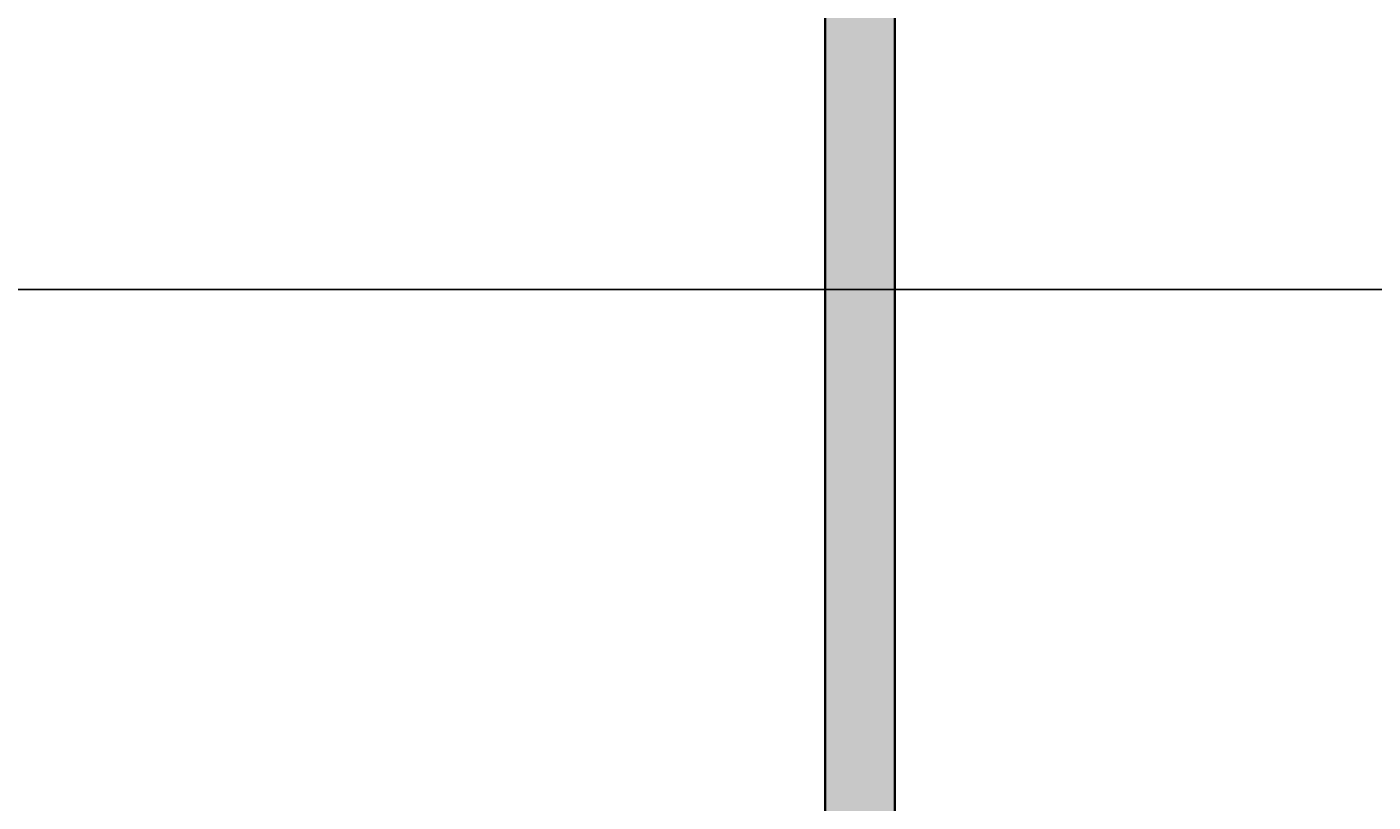
# Model space of a CAD drawing. Units: inches. Extents: x 1998 to 2588, y 1139 to 1977.
# Tile 5 of 134: x 2036 to 2075, y 1598 to 1620. Entities that reach past the tile are written whole.
import ezdxf

# ---------------------------------------------------------------- set-up
doc = ezdxf.new("R2010")
doc.units = ezdxf.units.IN
for name, color, linetype, lineweight in [('A-ANNO-DIMS', 2, 'Continuous', 18), ('A-WALL-PATT', 252, 'Continuous', 13), ('WALL', 200, 'Continuous', 35)]:
    doc.layers.add(name, color=color, linetype=linetype, lineweight=lineweight)
doc.styles.get("Standard").update_dxf_attribs({"font": 'arial.ttf'})
doc.dimstyles.get("Standard").update_dxf_attribs({"dimtxt": 0.18, "dimasz": 0.18, "dimexe": 0.18, "dimexo": 0.0625, "dimgap": 0.09, "dimtad": 0, "dimtih": 1, "dimtoh": 1, "dimdec": 4, "dimzin": 0, "dimdsep": 46, "dimtxsty": 'Standard', "dimcen": 0.09, "dimadec": 0, "dimazin": 0, "dimtfac": 1, "dimtdec": 4, "dimtofl": 0, "dimtmove": 0, "dimatfit": 3, "dimfxl": 1, "dimtolj": 1, "dimtzin": 0, "dimarcsym": 0})

# ---------------------------------------------------------------- blocks, each defined once
blk = doc.blocks.new('*D30')
at = {"layer": 'A-ANNO-DIMS', "color": 0, "lineweight": -2, "transparency": 16777216}
for p, q in [((2407.91, 1636.732), (1997.843, 1636.732)), ((1998.023, 1636.552), (1998.023, 1615.913)), ((1998.023, 1594.912), (1998.023, 1615.552)), ((2407.91, 1594.732), (1997.843, 1594.732))]:
    blk.add_line(p, q, dxfattribs=at)
at = {"layer": 'A-ANNO-DIMS', "color": 0, "transparency": 16777216}
for points in [[(1997.993, 1636.552), (1998.053, 1636.552), (1998.023, 1636.732)], [(1997.993, 1594.912), (1998.053, 1594.912), (1998.023, 1594.732)]]:
    blk.add_solid(points, dxfattribs=at)
at = {"layer": 'Defpoints', "color": 0, "transparency": 16777216}
for p in [(1998.023, 1636.732), (2407.973, 1636.732), (2407.973, 1594.732)]:
    blk.add_point(p, dxfattribs=at)
at = {"layer": 'A-ANNO-DIMS', "color": 0, "transparency": 16777216, "insert": (1998.023, 1615.732), "char_height": 0.18, "attachment_point": 5}
blk.add_mtext('\\A1;42', dxfattribs=at)
blk = doc.blocks.new('*D35')
at = {"layer": 'A-ANNO-DIMS', "color": 0, "lineweight": -2, "transparency": 16777216}
for p, q in [((2148.392, 1612.732), (1997.843, 1612.732)), ((1998.023, 1612.552), (1998.023, 1600.913)), ((1998.023, 1588.912), (1998.023, 1600.552)), ((2148.392, 1588.732), (1997.843, 1588.732))]:
    blk.add_line(p, q, dxfattribs=at)
at = {"layer": 'A-ANNO-DIMS', "color": 0, "transparency": 16777216}
for points in [[(1997.993, 1612.552), (1998.053, 1612.552), (1998.023, 1612.732)], [(1997.993, 1588.912), (1998.053, 1588.912), (1998.023, 1588.732)]]:
    blk.add_solid(points, dxfattribs=at)
at = {"layer": 'Defpoints', "color": 0, "transparency": 16777216}
for p in [(1998.023, 1612.732), (2148.455, 1612.732), (2148.455, 1588.732)]:
    blk.add_point(p, dxfattribs=at)
at = {"layer": 'A-ANNO-DIMS', "color": 0, "transparency": 16777216, "insert": (1998.023, 1600.732), "char_height": 0.18, "attachment_point": 5}
blk.add_mtext('\\A1;24', dxfattribs=at)
blk = doc.blocks.new('*D38')
at = {"layer": 'A-ANNO-DIMS', "color": 0, "lineweight": -2, "transparency": 16777216}
for p, q in [((2197.387, 1663.247), (1997.843, 1663.247)), ((1998.023, 1663.067), (1998.023, 1638.171)), ((1998.023, 1612.912), (1998.023, 1637.808)), ((2197.387, 1612.732), (1997.843, 1612.732))]:
    blk.add_line(p, q, dxfattribs=at)
at = {"layer": 'A-ANNO-DIMS', "color": 0, "transparency": 16777216}
for points in [[(1997.993, 1663.067), (1998.053, 1663.067), (1998.023, 1663.247)], [(1997.993, 1612.912), (1998.053, 1612.912), (1998.023, 1612.732)]]:
    blk.add_solid(points, dxfattribs=at)
at = {"layer": 'Defpoints', "color": 0, "transparency": 16777216}
for p in [(1998.023, 1663.247), (2197.45, 1663.247), (2197.45, 1612.732)]:
    blk.add_point(p, dxfattribs=at)
at = {"layer": 'A-ANNO-DIMS', "color": 0, "transparency": 16777216, "insert": (1998.023, 1637.99), "char_height": 0.18, "attachment_point": 5}
blk.add_mtext('\\A1;50.51', dxfattribs=at)

msp = doc.modelspace()

# ---------------------------------------------------------------- hatches: boundary and pattern name
at = {"layer": 'A-WALL-PATT'}
h = msp.add_hatch(color=256, dxfattribs=at)
h.dxf.hatch_style = 1
h.paths.add_polyline_path([(2227.4729, 1911.2324), (2222.9729, 1911.2324), (2222.9729, 1888.7324), (2227.4729, 1888.7324)])
h.paths.add_polyline_path([(2236.4493, 1870.3636), (2236.4493, 1875.2324), (2234.4125, 1875.2324), (2234.4125, 1868.3278), (2227.4729, 1868.3278), (2227.4729, 1866.2324), (2236.4493, 1866.2324)])
h.paths.add_polyline_path([(2330.0332, 1875.2324), (2263.9907, 1875.2324), (2263.9907, 1866.2324), (2330.0332, 1866.2324)])
h.paths.add_polyline_path([(2345.9729, 1906.7324), (2393.9729, 1906.7324), (2393.9729, 1882.7324), (2345.9729, 1882.7324), (2345.9729, 1878.2324), (2393.9729, 1878.2324), (2398.4729, 1878.2324), (2398.4729, 1882.7324), (2398.4729, 1911.2324), (2345.9729, 1911.2324), (2341.4729, 1911.2324), (2341.4729, 1866.2324), (2341.4729, 1790.0412), (2345.9729, 1790.0412), (2345.9729, 1875.2324)])
h.paths.add_polyline_path([(2398.4729, 1878.2324), (2393.9729, 1878.2324), (2393.9729, 1798.2324), (2393.9729, 1793.7324), (2398.4729, 1793.7324)], flags=17)
h.paths.add_polyline_path([(2393.9729, 1798.2324), (2375.7311, 1798.2324, -0.005968), (2375.7384, 1797.6146), (2375.7384, 1793.7324), (2393.9729, 1793.7324)], flags=17)
h.paths.add_polyline_path([(2349.8569, 1797.6146), (2349.8569, 1798.2324), (2345.9729, 1798.2324), (2345.9729, 1793.7324), (2349.8569, 1793.7324)], flags=17)
h.paths.add_polyline_path([(2398.4729, 1793.7324), (2393.9729, 1793.7324), (2393.9729, 1790.0412), (2398.4729, 1790.0412)], flags=17)
h.paths.add_polyline_path([(2527.4729, 1882.7324), (2507.8006, 1882.7324), (2507.8006, 1878.2324), (2518.4729, 1878.2324), (2518.4729, 1759.7324), (2510.9729, 1759.7324), (2510.9729, 1755.2324), (2527.4729, 1755.2324)])
h.paths.add_polyline_path([(2487.396, 1882.7324), (2398.4729, 1882.7324), (2398.4729, 1878.2324), (2487.396, 1878.2324)])
h.paths.add_polyline_path([(2490.5682, 1759.7324), (2345.9729, 1759.7324), (2345.9729, 1755.2324), (2490.5682, 1755.2324)])
h.paths.add_polyline_path([(2398.4729, 1760.5844), (2398.3914, 1760.5844), (2393.9729, 1760.5844), (2393.9729, 1759.7324), (2398.4729, 1759.7324)])
h.paths.add_polyline_path([(2334.5332, 1759.7324), (2234.4125, 1759.7324), (2234.4125, 1755.2324), (2334.5332, 1755.2324)])
h.paths.add_polyline_path([(2345.9729, 1760.5844), (2341.5543, 1760.5844), (2341.4729, 1760.5844), (2341.4729, 1759.7324), (2345.9729, 1759.7324)])
h.paths.add_polyline_path([(2222.9729, 1759.7324), (2221.7204, 1759.7324), (2221.7204, 1755.2324), (2222.9729, 1755.2324)])
h.paths.add_polyline_path([(2061.4729, 1702.7324), (2059.4729, 1702.7324), (2059.4729, 1584.2324), (2061.4729, 1584.2324)])
h.paths.add_polyline_path([(2061.4729, 1584.2324), (2059.4729, 1584.2324), (2059.4729, 1470.2324), (2061.4729, 1470.2324)])
h.paths.add_polyline_path([(2510.9729, 1469.2927), (2501.9729, 1469.2927), (2501.9729, 1369.172), (2510.9729, 1369.172)])
h.paths.add_polyline_path([(2227.4729, 1369.7324), (2227.4729, 1417.7324), (2221.4126, 1417.7324), (2221.4126, 1413.2324), (2222.9729, 1413.2324), (2222.9729, 1293.2324), (2222.9729, 1285.137), (2227.4729, 1285.137)])

# ---------------------------------------------------------------- linework, layer by layer
at = {"layer": 'WALL'}
for p, q in [((2061.4729, 1473.2749), (2061.4729, 1705.7749)), ((2059.4729, 1470.2324), (2059.4729, 1702.7324))]:
    msp.add_line(p, q, dxfattribs=at)
msp.add_lwpolyline([(2059.4729, 1584.2324), (2061.4729, 1584.2324), (2061.4729, 1702.7324), (2059.4729, 1702.7324)], close=True, dxfattribs=at)

# ---------------------------------------------------------------- dimensions: what is measured, and where the dimension line sits
at = {"layer": 'A-ANNO-DIMS'}
for base, p1, p2, override, picture, middle in [((1998.0229, 1663.2466), (2197.4499, 1612.7324), (2197.4499, 1663.2466), {"dimdec": 2, "dimlfac": 1, "dimrnd": 0, "dimzin": 0, "dimdsep": 46, "dimlunit": 2}, '*D38', (1998.0229, 1637.9895)), ((1998.0229, 1636.7324), (2407.9729, 1594.7324), (2407.9729, 1636.7324), {"dimdec": 0, "dimlfac": 1, "dimrnd": 0, "dimzin": 0, "dimdsep": 46, "dimlunit": 2}, '*D30', (1998.0229, 1615.7324)), ((1998.0229, 1612.7324), (2148.4548, 1588.7324), (2148.4548, 1612.7324), {"dimdec": 0, "dimlfac": 1, "dimrnd": 0, "dimzin": 0, "dimdsep": 46, "dimlunit": 2}, '*D35', (1998.0229, 1600.7324))]:
    dim = msp.add_linear_dim(base=base, p1=p1, p2=p2, angle=90, dimstyle='Standard', override=override, dxfattribs=at)
    dim.commit()
    dim.dimension.update_dxf_attribs({"geometry": picture, "text_midpoint": middle})

doc.saveas('drawing.dxf')
